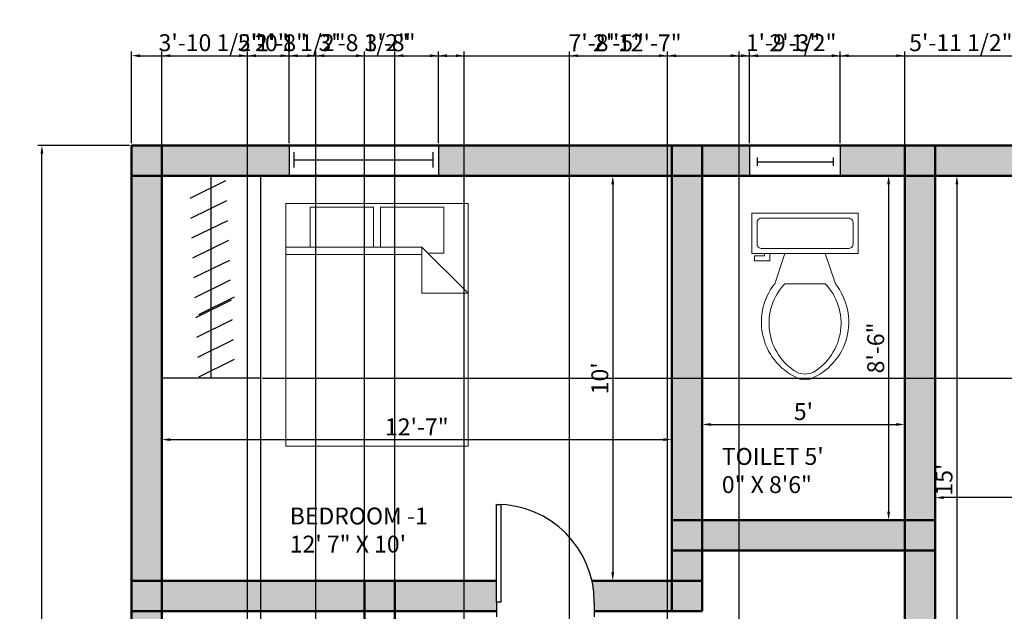
# Model space of a CAD drawing. Units: millimetres. Extents: x 2976 to 3516, y 849 to 1445.
# Tile 5 of 7: x 2981 to 3272, y 1270 to 1445. Entities that reach past the tile are written whole.
import ezdxf

# ---------------------------------------------------------------- set-up
doc = ezdxf.new("R2010")
doc.units = ezdxf.units.MM
for name, color, linetype, lineweight in [('A-AREA-IDEN', 150, 'Continuous', 25), ('A-FLOR-CASE', 130, 'Continuous', 25), ('A-FLOR-FIXT', 130, 'Continuous', 18), ('A-WALL-PATT', 3, 'Continuous', 13), ('dimensions', 50, 'Continuous', 18), ('doors', 190, 'Continuous', 25), ('furniture', 130, 'Continuous', 18), ('walls', 80, 'Continuous', 50), ('windows', 10, 'Continuous', 25)]:
    doc.layers.add(name, color=color, linetype=linetype, lineweight=lineweight)
doc.styles.get("Standard").update_dxf_attribs({"font": 'arial.ttf'})
doc.dimstyles.new('ISO-25', dxfattribs={"dimtxt": 5, "dimasz": 2.5, "dimexe": 1.25, "dimexo": 0.625, "dimtad": 1, "dimdec": 0, "dimlunit": 3, "dimtxsty": 'Standard', "dimcen": 2.5, "dimadec": 0, "dimazin": 0, "dimtfac": 1, "dimtdec": 0, "dimtmove": 0, "dimatfit": 3, "dimfxl": 1, "dimarcsym": 0})

# ---------------------------------------------------------------- blocks, each defined once
blk = doc.blocks.new('*U2')
for p, q in [((0, 0), (0, -6)), ((40, 0), (40, -6))]:
    blk.add_line(p, q)
blk.add_lwpolyline([(0, 0), (0, 40), (1.75, 40), (1.75, 0)], close=True)
blk.add_arc((0, 0), 40, 0, 90)
blk = doc.blocks.new('*U4')
for p, q in [((0, 4), (0, 0)), ((36, 4), (36, 0)), ((0, 2), (36, 2))]:
    blk.add_line(p, q)
blk = doc.blocks.new('*U5')
for p, q in [((0, 4), (0, 0)), ((0, 2), (36, 2)), ((36, 4), (36, 0))]:
    blk.add_line(p, q)
blk = doc.blocks.new('Bed - Queen')
for p, q in [((0, -80.00003), (0, 0)), ((0, 0), (59.99999, 0)), ((59.99999, 0), (59.99999, -80.00003)), ((7.99999, -1.2), (28.79998, -1.2)), ((7.99999, -14.4), (7.99999, -1.2)), ((28.79998, -1.2), (28.79998, -14.4)), ((31.19999, -1.2), (51.99999, -1.2)), ((31.19999, -14.4), (31.19999, -1.2)), ((51.99999, -1.2), (51.99999, -16.4)), ((0, -14.4), (44.8, -14.4)), ((59.99999, -29.6), (44.8, -14.4)), ((44.8, -14.4), (44.8, -29.6)), ((44.8, -16.8), (0, -16.8)), ((51.99999, -16.4), (46.79936, -16.4)), ((44.8, -29.6), (59.99999, -29.6)), ((59.99999, -80.00003), (0, -80.00003))]:
    blk.add_line(p, q)
blk = doc.blocks.new('Toilet - top')
for p, q in [((9.5, -6), (9.5, -2)), ((-10, -8.5), (-8, -8.5)), ((-10, -9.5), (-10, -8.5)), ((-7, -9.5), (-10, -9.5)), ((-8, -8.5), (-8, -8)), ((-7, -8), (-7, -9.5)), ((-4, -8), (-6, -14)), ((4, -8), (6, -14)), ((4, -14), (-4, -14))]:
    blk.add_line(p, q)
blk.add_lwpolyline([(10.5, -8), (10.5, 0), (-10.5, 0), (-10.5, -8)], close=True)
for points in [[(8.5, -1), (-8.5, -1)], [(-9.5, -2), (-9.5, -6)], [(-8.5, -7), (8.5, -7)]]:
    blk.add_lwpolyline(points)
for centre, radius, start, end in [((-8.62, -1.88), 0.884, 81.8699, 188.1301), ((8.62, -1.88), 0.884, 351.8699, 98.1301), ((-8.62, -6.12), 0.884, 171.8699, 278.1301), ((8.62, -6.12), 0.884, 261.8699, 8.1301), ((3.52, -21.58), 12.17, 141.4691, 247.9714), ((4.2, -21.82), 11.33, 136.3677, 238.9468), ((-3.52, -21.58), 12.17, 292.0284, 38.5307), ((-4.2, -21.82), 11.33, 301.053, 43.6321), ((0, -27.88), 4, 245.7318, 294.2682), ((0, -29), 4, 254.8605, 285.1395)]:
    blk.add_arc(centre, radius, start, end)
blk = doc.blocks.new('*D9')
at = {"layer": 'Defpoints', "color": 0, "transparency": 16777216}
for p in [(3156.2, 1398.88), (3156.2, 1278.88), (3156.2, 1278.88)]:
    blk.add_point(p, dxfattribs=at)
at = {"layer": 'dimensions', "color": 0, "lineweight": -2, "transparency": 16777216}
for p, q in [((3156.83, 1398.88), (3157.45, 1398.88)), ((3156.2, 1396.38), (3156.2, 1281.38)), ((3156.83, 1278.88), (3157.45, 1278.88))]:
    blk.add_line(p, q, dxfattribs=at)
at = {"layer": 'dimensions', "color": 0, "transparency": 16777216}
for points in [[(3155.78, 1396.38), (3156.62, 1396.38), (3156.2, 1398.88)], [(3155.78, 1281.38), (3156.62, 1281.38), (3156.2, 1278.88)]]:
    blk.add_solid(points, dxfattribs=at)
at = {"layer": 'dimensions', "color": 0, "transparency": 16777216, "insert": (3153.02, 1338.88), "char_height": 5, "attachment_point": 5, "rotation": 90}
blk.add_mtext("10'", dxfattribs=at)
blk = doc.blocks.new('*D10')
at = {"layer": 'Defpoints', "color": 0, "transparency": 16777216}
for p in [(3173.67, 1320.72), (3022.67, 1317.67), (3173.67, 1317.67)]:
    blk.add_point(p, dxfattribs=at)
at = {"layer": 'dimensions', "color": 0, "lineweight": -2, "transparency": 16777216}
for p, q in [((3022.67, 1318.3), (3022.67, 1321.97)), ((3173.67, 1318.3), (3173.67, 1321.97)), ((3025.17, 1320.72), (3171.17, 1320.72))]:
    blk.add_line(p, q, dxfattribs=at)
at = {"layer": 'dimensions', "color": 0, "transparency": 16777216}
for points in [[(3025.17, 1321.14), (3025.17, 1320.31), (3022.67, 1320.72)], [(3171.17, 1321.14), (3171.17, 1320.31), (3173.67, 1320.72)]]:
    blk.add_solid(points, dxfattribs=at)
at = {"layer": 'dimensions', "color": 0, "transparency": 16777216, "insert": (3098.17, 1323.86), "char_height": 5, "attachment_point": 5}
blk.add_mtext('12\'-7"', dxfattribs=at)
blk = doc.blocks.new('*D11')
at = {"layer": 'Defpoints', "color": 0, "transparency": 16777216}
for p in [(3237.91, 1398.88), (3237.91, 1296.88), (3237.91, 1296.88)]:
    blk.add_point(p, dxfattribs=at)
at = {"layer": 'dimensions', "color": 0, "lineweight": -2, "transparency": 16777216}
for p, q in [((3238.54, 1398.88), (3239.16, 1398.88)), ((3237.91, 1396.38), (3237.91, 1299.38)), ((3238.54, 1296.88), (3239.16, 1296.88))]:
    blk.add_line(p, q, dxfattribs=at)
at = {"layer": 'dimensions', "color": 0, "transparency": 16777216}
for points in [[(3237.49, 1396.38), (3238.33, 1396.38), (3237.91, 1398.88)], [(3237.49, 1299.38), (3238.33, 1299.38), (3237.91, 1296.88)]]:
    blk.add_solid(points, dxfattribs=at)
at = {"layer": 'dimensions', "color": 0, "transparency": 16777216, "insert": (3234.73, 1347.88), "char_height": 5, "attachment_point": 5, "rotation": 90}
blk.add_mtext('8\'-6"', dxfattribs=at)
blk = doc.blocks.new('*D12')
at = {"layer": 'Defpoints', "color": 0, "transparency": 16777216}
for p in [(3242.67, 1325.21), (3182.67, 1321.08), (3242.67, 1321.08)]:
    blk.add_point(p, dxfattribs=at)
at = {"layer": 'dimensions', "color": 0, "lineweight": -2, "transparency": 16777216}
for p, q in [((3182.67, 1321.71), (3182.67, 1326.46)), ((3185.17, 1325.21), (3240.17, 1325.21)), ((3242.67, 1321.71), (3242.67, 1326.46))]:
    blk.add_line(p, q, dxfattribs=at)
at = {"layer": 'dimensions', "color": 0, "transparency": 16777216}
for points in [[(3185.17, 1325.63), (3185.17, 1324.79), (3182.67, 1325.21)], [(3240.17, 1325.63), (3240.17, 1324.79), (3242.67, 1325.21)]]:
    blk.add_solid(points, dxfattribs=at)
at = {"layer": 'dimensions', "color": 0, "transparency": 16777216, "insert": (3212.67, 1328.38), "char_height": 5, "attachment_point": 5}
blk.add_mtext("5'", dxfattribs=at)
blk = doc.blocks.new('*D13')
at = {"layer": 'Defpoints', "color": 0, "transparency": 16777216}
for p in [(3251.67, 1303.56), (3251.67, 1303.56), (3383.67, 1303.56)]:
    blk.add_point(p, dxfattribs=at)
at = {"layer": 'dimensions', "color": 0, "lineweight": -2, "transparency": 16777216}
for p, q in [((3251.67, 1304.18), (3251.67, 1304.81)), ((3383.67, 1304.18), (3383.67, 1304.81)), ((3381.17, 1303.56), (3254.17, 1303.56))]:
    blk.add_line(p, q, dxfattribs=at)
at = {"layer": 'dimensions', "color": 0, "transparency": 16777216}
for points in [[(3254.17, 1303.98), (3254.17, 1303.14), (3251.67, 1303.56)], [(3381.17, 1303.98), (3381.17, 1303.14), (3383.67, 1303.56)]]:
    blk.add_solid(points, dxfattribs=at)
at = {"layer": 'dimensions', "color": 0, "transparency": 16777216, "insert": (3317.67, 1306.69), "char_height": 5, "attachment_point": 5}
blk.add_mtext("11'", dxfattribs=at)
blk = doc.blocks.new('*D14')
at = {"layer": 'Defpoints', "color": 0, "transparency": 16777216}
for p in [(3258.13, 1398.88), (3258.13, 1218.88), (3258.13, 1218.88)]:
    blk.add_point(p, dxfattribs=at)
at = {"layer": 'dimensions', "color": 0, "lineweight": -2, "transparency": 16777216}
for p, q in [((3258.76, 1398.88), (3259.38, 1398.88)), ((3258.13, 1396.38), (3258.13, 1221.38)), ((3258.76, 1218.88), (3259.38, 1218.88))]:
    blk.add_line(p, q, dxfattribs=at)
at = {"layer": 'dimensions', "color": 0, "transparency": 16777216}
for points in [[(3257.72, 1396.38), (3258.55, 1396.38), (3258.13, 1398.88)], [(3257.72, 1221.38), (3258.55, 1221.38), (3258.13, 1218.88)]]:
    blk.add_solid(points, dxfattribs=at)
at = {"layer": 'dimensions', "color": 0, "transparency": 16777216, "insert": (3254.96, 1308.88), "char_height": 5, "attachment_point": 5, "rotation": 90}
blk.add_mtext("15'", dxfattribs=at)
blk = doc.blocks.new('*D39')
at = {"layer": 'Defpoints', "color": 0, "transparency": 16777216}
for p in [(2987.13, 1407.88), (3013.67, 1407.88), (3013.67, 879.88)]:
    blk.add_point(p, dxfattribs=at)
at = {"layer": 'dimensions', "color": 0, "lineweight": -2, "transparency": 16777216}
for p, q in [((3013.05, 1407.88), (2985.88, 1407.88)), ((2987.13, 882.38), (2987.13, 1405.38)), ((3013.05, 879.88), (2985.88, 879.88))]:
    blk.add_line(p, q, dxfattribs=at)
at = {"layer": 'dimensions', "color": 0, "transparency": 16777216}
for points in [[(2986.71, 1405.38), (2987.55, 1405.38), (2987.13, 1407.88)], [(2986.71, 882.38), (2987.55, 882.38), (2987.13, 879.88)]]:
    blk.add_solid(points, dxfattribs=at)
at = {"layer": 'dimensions', "color": 0, "transparency": 16777216, "insert": (2983.95, 1143.88), "char_height": 5, "attachment_point": 5, "rotation": 90}
blk.add_mtext('44\'-0"', dxfattribs=at)
blk = doc.blocks.new('*D43')
at = {"layer": 'Defpoints', "color": 0, "transparency": 16777216}
for p in [(3082.67, 1434.42), (3022.67, 1140.88), (3082.67, 1140.88)]:
    blk.add_point(p, dxfattribs=at)
at = {"layer": 'dimensions', "color": 0, "lineweight": -2, "transparency": 16777216}
for p, q in [((3022.67, 1141.51), (3022.67, 1435.67)), ((3082.67, 1141.51), (3082.67, 1435.67)), ((3025.17, 1434.42), (3080.17, 1434.42))]:
    blk.add_line(p, q, dxfattribs=at)
at = {"layer": 'dimensions', "color": 0, "transparency": 16777216}
for points in [[(3025.17, 1434.84), (3025.17, 1434), (3022.67, 1434.42)], [(3080.17, 1434.84), (3080.17, 1434), (3082.67, 1434.42)]]:
    blk.add_solid(points, dxfattribs=at)
at = {"layer": 'dimensions', "color": 0, "transparency": 16777216, "insert": (3052.67, 1437.6), "char_height": 5, "attachment_point": 5}
blk.add_mtext('5\'-0"', dxfattribs=at)
blk = doc.blocks.new('*D44')
at = {"layer": 'Defpoints', "color": 0, "transparency": 16777216}
for p in [(3242.67, 1434.42), (3091.67, 1224.53), (3242.67, 1209.88)]:
    blk.add_point(p, dxfattribs=at)
at = {"layer": 'dimensions', "color": 0, "lineweight": -2, "transparency": 16777216}
for p, q in [((3091.67, 1225.16), (3091.67, 1435.67)), ((3242.67, 1210.51), (3242.67, 1435.67)), ((3094.17, 1434.42), (3240.17, 1434.42))]:
    blk.add_line(p, q, dxfattribs=at)
at = {"layer": 'dimensions', "color": 0, "transparency": 16777216}
for points in [[(3094.17, 1434.84), (3094.17, 1434), (3091.67, 1434.42)], [(3240.17, 1434.84), (3240.17, 1434), (3242.67, 1434.42)]]:
    blk.add_solid(points, dxfattribs=at)
at = {"layer": 'dimensions', "color": 0, "transparency": 16777216, "insert": (3167.17, 1437.56), "char_height": 5, "attachment_point": 5}
blk.add_mtext('12\'-7"', dxfattribs=at)
blk = doc.blocks.new('*D45')
at = {"layer": 'Defpoints', "color": 0, "transparency": 16777216}
for p in [(3060.33, 1434.42), (3013.67, 1407.88), (3060.33, 1407.88)]:
    blk.add_point(p, dxfattribs=at)
at = {"layer": 'dimensions', "color": 0, "lineweight": -2, "transparency": 16777216}
for p, q in [((3013.67, 1408.51), (3013.67, 1435.67)), ((3060.33, 1408.51), (3060.33, 1435.67)), ((3016.17, 1434.42), (3057.83, 1434.42))]:
    blk.add_line(p, q, dxfattribs=at)
at = {"layer": 'dimensions', "color": 0, "transparency": 16777216}
for points in [[(3016.17, 1434.84), (3016.17, 1434), (3013.67, 1434.42)], [(3057.83, 1434.84), (3057.83, 1434), (3060.33, 1434.42)]]:
    blk.add_solid(points, dxfattribs=at)
at = {"layer": 'dimensions', "color": 0, "transparency": 16777216, "insert": (3037, 1437.63), "char_height": 5, "attachment_point": 5}
blk.add_mtext('3\'-10 1/2"', dxfattribs=at)
blk = doc.blocks.new('*D46')
at = {"layer": 'Defpoints', "color": 0, "transparency": 16777216}
for p in [(3104.59, 1434.42), (3060.33, 1407.88), (3104.59, 1407.88)]:
    blk.add_point(p, dxfattribs=at)
at = {"layer": 'dimensions', "color": 0, "lineweight": -2, "transparency": 16777216}
for p, q in [((3060.33, 1408.51), (3060.33, 1435.67)), ((3104.59, 1408.51), (3104.59, 1435.67)), ((3062.83, 1434.42), (3102.09, 1434.42))]:
    blk.add_line(p, q, dxfattribs=at)
at = {"layer": 'dimensions', "color": 0, "transparency": 16777216}
for points in [[(3062.83, 1434.84), (3062.83, 1434), (3060.33, 1434.42)], [(3102.09, 1434.84), (3102.09, 1434), (3104.59, 1434.42)]]:
    blk.add_solid(points, dxfattribs=at)
at = {"layer": 'dimensions', "color": 0, "transparency": 16777216, "insert": (3082.46, 1437.63), "char_height": 5, "attachment_point": 5}
blk.add_mtext('3\'-8 1/2"', dxfattribs=at)
blk = doc.blocks.new('*D47')
at = {"layer": 'Defpoints', "color": 0, "transparency": 16777216}
for p in [(3196.7, 1434.42), (3104.59, 1407.88), (3196.7, 1407.88)]:
    blk.add_point(p, dxfattribs=at)
at = {"layer": 'dimensions', "color": 0, "lineweight": -2, "transparency": 16777216}
for p, q in [((3104.59, 1408.51), (3104.59, 1435.67)), ((3196.7, 1408.51), (3196.7, 1435.67)), ((3107.09, 1434.42), (3194.2, 1434.42))]:
    blk.add_line(p, q, dxfattribs=at)
at = {"layer": 'dimensions', "color": 0, "transparency": 16777216}
for points in [[(3107.09, 1434.84), (3107.09, 1434), (3104.59, 1434.42)], [(3194.2, 1434.84), (3194.2, 1434), (3196.7, 1434.42)]]:
    blk.add_solid(points, dxfattribs=at)
at = {"layer": 'dimensions', "color": 0, "transparency": 16777216, "insert": (3150.64, 1437.6), "char_height": 5, "attachment_point": 5}
blk.add_mtext('7\'-8"', dxfattribs=at)
blk = doc.blocks.new('*D48')
at = {"layer": 'Defpoints', "color": 0, "transparency": 16777216}
for p in [(3223.57, 1434.42), (3196.7, 1407.88), (3223.57, 1407.88)]:
    blk.add_point(p, dxfattribs=at)
at = {"layer": 'dimensions', "color": 0, "lineweight": -2, "transparency": 16777216}
for p, q in [((3196.7, 1408.51), (3196.7, 1435.67)), ((3223.57, 1408.51), (3223.57, 1435.67)), ((3199.2, 1434.42), (3221.07, 1434.42))]:
    blk.add_line(p, q, dxfattribs=at)
at = {"layer": 'dimensions', "color": 0, "transparency": 16777216}
for points in [[(3199.2, 1434.84), (3199.2, 1434), (3196.7, 1434.42)], [(3221.07, 1434.84), (3221.07, 1434), (3223.57, 1434.42)]]:
    blk.add_solid(points, dxfattribs=at)
at = {"layer": 'dimensions', "color": 0, "transparency": 16777216, "insert": (3210.14, 1437.6), "char_height": 5, "attachment_point": 5}
blk.add_mtext('2\'-3"', dxfattribs=at)
blk = doc.blocks.new('*D49')
at = {"layer": 'Defpoints', "color": 0, "transparency": 16777216}
for p in [(3295.02, 1434.42), (3223.57, 1407.88), (3295.02, 1407.88)]:
    blk.add_point(p, dxfattribs=at)
at = {"layer": 'dimensions', "color": 0, "lineweight": -2, "transparency": 16777216}
for p, q in [((3223.57, 1408.51), (3223.57, 1435.67)), ((3295.02, 1408.51), (3295.02, 1435.67)), ((3226.07, 1434.42), (3292.52, 1434.42))]:
    blk.add_line(p, q, dxfattribs=at)
at = {"layer": 'dimensions', "color": 0, "transparency": 16777216}
for points in [[(3226.07, 1434.84), (3226.07, 1434), (3223.57, 1434.42)], [(3292.52, 1434.84), (3292.52, 1434), (3295.02, 1434.42)]]:
    blk.add_solid(points, dxfattribs=at)
at = {"layer": 'dimensions', "color": 0, "transparency": 16777216, "insert": (3259.3, 1437.63), "char_height": 5, "attachment_point": 5}
blk.add_mtext('5\'-11 1/2"', dxfattribs=at)
blk = doc.blocks.new('*D54')
at = {"layer": 'Defpoints', "color": 0, "transparency": 16777216}
for p in [(3172.4, 1434.42), (3143.42, 1149.88), (3172.4, 1149.88)]:
    blk.add_point(p, dxfattribs=at)
at = {"layer": 'dimensions', "color": 0, "lineweight": -2, "transparency": 16777216}
for p, q in [((3143.42, 1150.51), (3143.42, 1435.67)), ((3172.4, 1150.51), (3172.4, 1435.67)), ((3145.92, 1434.42), (3169.9, 1434.42))]:
    blk.add_line(p, q, dxfattribs=at)
at = {"layer": 'dimensions', "color": 0, "transparency": 16777216}
for points in [[(3145.92, 1434.84), (3145.92, 1434), (3143.42, 1434.42)], [(3169.9, 1434.84), (3169.9, 1434), (3172.4, 1434.42)]]:
    blk.add_solid(points, dxfattribs=at)
at = {"layer": 'dimensions', "color": 0, "transparency": 16777216, "insert": (3157.91, 1437.6), "char_height": 5, "attachment_point": 5}
blk.add_mtext('2\'-5"', dxfattribs=at)
blk = doc.blocks.new('*D57')
at = {"layer": 'Defpoints', "color": 0, "transparency": 16777216}
for p in [(3112.23, 1434.42), (3068.25, 1017.88), (3112.23, 1017.88)]:
    blk.add_point(p, dxfattribs=at)
at = {"layer": 'dimensions', "color": 0, "lineweight": -2, "transparency": 16777216}
for p, q in [((3068.25, 1018.51), (3068.25, 1435.67)), ((3112.23, 1018.51), (3112.23, 1435.67)), ((3070.75, 1434.42), (3109.73, 1434.42))]:
    blk.add_line(p, q, dxfattribs=at)
at = {"layer": 'dimensions', "color": 0, "transparency": 16777216}
for points in [[(3070.75, 1434.84), (3070.75, 1434), (3068.25, 1434.42)], [(3109.73, 1434.84), (3109.73, 1434), (3112.23, 1434.42)]]:
    blk.add_solid(points, dxfattribs=at)
at = {"layer": 'dimensions', "color": 0, "transparency": 16777216, "insert": (3090.24, 1437.6), "char_height": 5, "attachment_point": 5}
blk.add_mtext('3\'-8"', dxfattribs=at)
blk = doc.blocks.new('*D73')
at = {"layer": 'Defpoints', "color": 0, "transparency": 16777216}
for p in [(3193.67, 1434.42), (3172.4, 1149.88), (3193.67, 1149.88)]:
    blk.add_point(p, dxfattribs=at)
at = {"layer": 'dimensions', "color": 0, "lineweight": -2, "transparency": 16777216}
for p, q in [((3172.4, 1150.51), (3172.4, 1435.67)), ((3193.67, 1150.51), (3193.67, 1435.67)), ((3174.9, 1434.42), (3191.17, 1434.42)), ((3193.67, 1434.42), (3221.89, 1434.42))]:
    blk.add_line(p, q, dxfattribs=at)
at = {"layer": 'dimensions', "color": 0, "transparency": 16777216}
for points in [[(3174.9, 1434.84), (3174.9, 1434), (3172.4, 1434.42)], [(3191.17, 1434.84), (3191.17, 1434), (3193.67, 1434.42)]]:
    blk.add_solid(points, dxfattribs=at)
at = {"layer": 'dimensions', "color": 0, "transparency": 16777216, "insert": (3209.03, 1437.63), "char_height": 5, "attachment_point": 5}
blk.add_mtext('1\'-9 1/2"', dxfattribs=at)
blk = doc.blocks.new('*D75')
at = {"layer": 'Defpoints', "color": 0, "transparency": 16777216}
for p in [(3022.67, 1338.88), (3051.83, 1338.88), (3051.83, 853.34)]:
    blk.add_point(p, dxfattribs=at)
at = {"layer": 'dimensions', "color": 0, "lineweight": -2, "transparency": 16777216}
for p, q in [((3022.67, 1338.26), (3022.67, 852.09)), ((3051.83, 1338.26), (3051.83, 852.09)), ((3025.17, 853.34), (3049.33, 853.34))]:
    blk.add_line(p, q, dxfattribs=at)
at = {"layer": 'dimensions', "color": 0, "transparency": 16777216}
for points in [[(3025.17, 853.76), (3025.17, 852.92), (3022.67, 853.34)], [(3049.33, 853.76), (3049.33, 852.92), (3051.83, 853.34)]]:
    blk.add_solid(points, dxfattribs=at)
at = {"layer": 'dimensions', "color": 0, "transparency": 16777216, "insert": (3037.25, 856.52), "char_height": 5, "attachment_point": 5}
blk.add_mtext('2\'-5"', dxfattribs=at)
blk = doc.blocks.new('*D76')
at = {"layer": 'Defpoints', "color": 0, "transparency": 16777216}
for p in [(3051.83, 1398.88), (3512.21, 1398.88), (3051.83, 1338.88)]:
    blk.add_point(p, dxfattribs=at)
at = {"layer": 'dimensions', "color": 0, "lineweight": -2, "transparency": 16777216}
for p, q in [((3052.46, 1398.88), (3513.46, 1398.88)), ((3512.21, 1341.38), (3512.21, 1396.38)), ((3052.46, 1338.88), (3513.46, 1338.88))]:
    blk.add_line(p, q, dxfattribs=at)
at = {"layer": 'dimensions', "color": 0, "transparency": 16777216}
for points in [[(3511.79, 1396.38), (3512.63, 1396.38), (3512.21, 1398.88)], [(3511.79, 1341.38), (3512.63, 1341.38), (3512.21, 1338.88)]]:
    blk.add_solid(points, dxfattribs=at)
at = {"layer": 'dimensions', "color": 0, "transparency": 16777216, "insert": (3509.03, 1368.88), "char_height": 5, "attachment_point": 5, "rotation": 90}
blk.add_mtext('5\'-0"', dxfattribs=at)
blk = doc.blocks.new('*D77')
at = {"layer": 'Defpoints', "color": 0, "transparency": 16777216}
for p in [(3048, 1434.42), (3022.67, 1079.38), (3048, 1079.38)]:
    blk.add_point(p, dxfattribs=at)
at = {"layer": 'dimensions', "color": 0, "lineweight": -2, "transparency": 16777216}
for p, q in [((3022.67, 1080.01), (3022.67, 1435.67)), ((3048, 1080.01), (3048, 1435.67)), ((3025.17, 1434.42), (3045.5, 1434.42)), ((3048, 1434.42), (3076.78, 1434.42))]:
    blk.add_line(p, q, dxfattribs=at)
at = {"layer": 'dimensions', "color": 0, "transparency": 16777216}
for points in [[(3025.17, 1434.84), (3025.17, 1434), (3022.67, 1434.42)], [(3045.5, 1434.84), (3045.5, 1434), (3048, 1434.42)]]:
    blk.add_solid(points, dxfattribs=at)
at = {"layer": 'dimensions', "color": 0, "transparency": 16777216, "insert": (3063.64, 1437.63), "char_height": 5, "attachment_point": 5}
blk.add_mtext('2\'-1 1/2"', dxfattribs=at)
blk = doc.blocks.new('*D79')
at = {"layer": 'Defpoints', "color": 0, "transparency": 16777216}
for p in [(3068.25, 1434.42), (3048, 1017.88), (3068.25, 1017.88)]:
    blk.add_point(p, dxfattribs=at)
at = {"layer": 'dimensions', "color": 0, "lineweight": -2, "transparency": 16777216}
for p, q in [((3048, 1018.51), (3048, 1435.67)), ((3068.25, 1018.51), (3068.25, 1435.67)), ((3050.5, 1434.42), (3065.75, 1434.42))]:
    blk.add_line(p, q, dxfattribs=at)
at = {"layer": 'dimensions', "color": 0, "transparency": 16777216}
for points in [[(3050.5, 1434.84), (3050.5, 1434), (3048, 1434.42)], [(3065.75, 1434.84), (3065.75, 1434), (3068.25, 1434.42)]]:
    blk.add_solid(points, dxfattribs=at)
at = {"layer": 'dimensions', "color": 0, "transparency": 16777216, "insert": (3058.12, 1437.6), "char_height": 5, "attachment_point": 5}
blk.add_mtext('1\'-8"', dxfattribs=at)

msp = doc.modelspace()

# ---------------------------------------------------------------- hatches: boundary and pattern name
at = {"layer": 'A-WALL-PATT'}
h = msp.add_hatch(color=256, dxfattribs=at)
h.dxf.hatch_style = 1
h.paths.add_polyline_path([(3022.67, 1398.88), (3013.67, 1398.88), (3013.67, 1278.88), (3022.67, 1278.88)])
h.paths.add_polyline_path([(3082.67, 1278.88), (3022.67, 1278.88), (3022.67, 1269.88), (3082.67, 1269.88)])
h.paths.add_polyline_path([(3022.67, 1278.88), (3013.67, 1278.88), (3013.67, 1269.88), (3022.67, 1269.88)])
h.paths.add_polyline_path([(3091.67, 1278.88), (3082.67, 1278.88), (3082.67, 1269.88), (3091.67, 1269.88)])
h.paths.add_polyline_path([(3121.76, 1278.88), (3091.67, 1278.88), (3091.67, 1269.88), (3121.76, 1269.88), (3121.76, 1272.56)])
h.paths.add_polyline_path([(3022.67, 1269.88), (3013.67, 1269.88), (3013.67, 1149.88), (3022.67, 1149.88)])
h.paths.add_polyline_path([(3022.67, 1140.88), (3013.67, 1140.88), (3013.67, 1017.88), (3022.67, 1017.88)])
h.paths.add_polyline_path([(3022.67, 1149.88), (3013.67, 1149.88), (3013.67, 1140.88), (3022.67, 1140.88)])
h.paths.add_polyline_path([(3082.67, 1149.88), (3022.67, 1149.88), (3022.67, 1140.88), (3082.67, 1140.88)])
h.paths.add_polyline_path([(3091.67, 1149.88), (3082.67, 1149.88), (3082.67, 1140.88), (3091.67, 1140.88)])
h.paths.add_polyline_path([(3143.42, 1147.68), (3143.42, 1149.88), (3091.67, 1149.88), (3091.67, 1140.88), (3144.23, 1140.88, -0.059251)])
h.paths.add_polyline_path([(3193.67, 1149.88), (3172.4, 1149.88), (3172.4, 1147.68), (3172.4, 1140.88), (3193.67, 1140.88)])
h.paths.add_polyline_path([(3202.67, 1149.88), (3193.67, 1149.88), (3193.67, 1140.88), (3202.67, 1140.88)])
h.paths.add_polyline_path([(3272.67, 1149.88), (3262.67, 1149.88), (3262.67, 1140.88), (3272.67, 1140.88)])
h.paths.add_polyline_path([(3272.67, 1140.88), (3262.67, 1140.88), (3262.67, 1083.88), (3272.67, 1083.88)])
h.paths.add_polyline_path([(3202.67, 1140.88), (3193.67, 1140.88), (3193.67, 1090.58), (3195.4, 1090.58, -0.118064), (3202.67, 1088.84)])
h.paths.add_polyline_path([(3202.67, 1074.53), (3195.4, 1074.53), (3193.67, 1074.53), (3193.67, 1017.88), (3202.67, 1017.88)])
h.paths.add_polyline_path([(3202.67, 1017.88), (3193.67, 1017.88), (3193.67, 1008.88), (3202.67, 1008.88)])
h.paths.add_polyline_path([(3193.67, 1017.88), (3112.23, 1017.88), (3112.23, 1008.88), (3193.67, 1008.88)])
h.paths.add_polyline_path([(3068.25, 1017.88), (3022.67, 1017.88), (3022.67, 1008.88), (3068.25, 1008.88)])
h.paths.add_polyline_path([(3022.67, 1017.88), (3013.67, 1017.88), (3013.67, 1008.88), (3022.67, 1008.88)])
h.paths.add_polyline_path([(3272.67, 1074.88), (3262.67, 1074.88), (3262.67, 1017.88), (3271.67, 1017.88), (3272.67, 1017.88)])
h.paths.add_polyline_path([(3272.67, 1083.88), (3262.67, 1083.88), (3262.67, 1074.88), (3272.67, 1074.88)])
h.paths.add_polyline_path([(3284.41, 1082.91), (3284.41, 1083.88), (3272.67, 1083.88), (3272.67, 1074.88), (3284.41, 1074.88)])
h.paths.add_polyline_path([(3383.67, 1083.88), (3300.46, 1083.88), (3300.46, 1082.91, -0.131652), (3298.31, 1074.88), (3383.67, 1074.88)])
h.paths.add_polyline_path([(3392.67, 1083.88), (3383.67, 1083.88), (3383.67, 1074.88), (3392.67, 1074.88)])
h.paths.add_polyline_path([(3392.67, 1074.88), (3383.67, 1074.88), (3383.67, 1017.88), (3392.67, 1017.88)])
h.paths.add_polyline_path([(3392.67, 1017.88), (3383.67, 1017.88), (3383.67, 1008.88), (3392.67, 1008.88)])
h.paths.add_polyline_path([(3383.67, 1017.88), (3347.17, 1017.88), (3347.17, 1008.88), (3383.67, 1008.88)])
h.paths.add_polyline_path([(3303.78, 1017.88), (3272.67, 1017.88), (3272.67, 1008.88), (3303.78, 1008.88)])
h.paths.add_polyline_path([(3272.67, 1017.88), (3271.67, 1017.88), (3262.67, 1017.88), (3262.67, 1008.88), (3272.67, 1008.88)])
h.paths.add_polyline_path([(3262.67, 1017.88), (3243.44, 1017.88), (3243.44, 1008.88), (3262.67, 1008.88)])
h.paths.add_polyline_path([(3218.58, 1017.88), (3202.67, 1017.88), (3202.67, 1008.88), (3218.58, 1008.88)])
h.paths.add_polyline_path([(3392.67, 1209.88), (3383.67, 1209.88), (3383.67, 1083.88), (3392.67, 1083.88)])
h.paths.add_polyline_path([(3392.67, 1218.88), (3383.67, 1218.88), (3383.67, 1209.88), (3392.67, 1209.88)])
h.paths.add_polyline_path([(3392.67, 1246.1), (3383.67, 1246.1), (3383.67, 1218.88), (3392.67, 1218.88)])
h.paths.add_polyline_path([(3383.67, 1218.88), (3251.67, 1218.88), (3251.67, 1209.88), (3383.67, 1209.88)])
h.paths.add_polyline_path([(3251.67, 1287.88), (3242.67, 1287.88), (3242.67, 1218.88), (3251.67, 1218.88)])
h.paths.add_polyline_path([(3251.67, 1218.88), (3242.67, 1218.88), (3242.67, 1209.88), (3251.67, 1209.88)])
h.paths.add_polyline_path([(3251.67, 1398.88), (3242.67, 1398.88), (3242.67, 1296.88), (3251.67, 1296.88)])
h.paths.add_polyline_path([(3251.67, 1296.88), (3242.67, 1296.88), (3242.67, 1287.88), (3251.67, 1287.88)])
h.paths.add_polyline_path([(3242.67, 1296.88), (3182.67, 1296.88), (3182.67, 1287.88), (3242.67, 1287.88)])
h.paths.add_polyline_path([(3182.67, 1296.88), (3173.67, 1296.88), (3173.67, 1287.88), (3182.67, 1287.88)])
h.paths.add_polyline_path([(3182.67, 1287.88), (3173.67, 1287.88), (3173.67, 1278.88), (3182.67, 1278.88)])
h.paths.add_polyline_path([(3182.67, 1278.88), (3173.67, 1278.88), (3173.67, 1269.88), (3182.67, 1269.88)])
h.paths.add_polyline_path([(3173.67, 1278.88), (3150.05, 1278.88, -0.054989), (3150.74, 1272.56), (3150.74, 1269.88), (3173.67, 1269.88)])
h.paths.add_polyline_path([(3182.67, 1398.88), (3173.67, 1398.88), (3173.67, 1296.88), (3182.67, 1296.88)])
h.paths.add_polyline_path([(3182.67, 1407.88), (3173.67, 1407.88), (3173.67, 1398.88), (3182.67, 1398.88)])
h.paths.add_polyline_path([(3173.67, 1407.88), (3104.59, 1407.88), (3104.59, 1398.88), (3173.67, 1398.88)])
h.paths.add_polyline_path([(3060.33, 1407.88), (3022.67, 1407.88), (3022.67, 1398.88), (3060.33, 1398.88)])
h.paths.add_polyline_path([(3022.67, 1407.88), (3013.67, 1407.88), (3013.67, 1398.88), (3022.67, 1398.88)])
h.paths.add_polyline_path([(3196.7, 1407.88), (3182.67, 1407.88), (3182.67, 1398.88), (3196.7, 1398.88)])
h.paths.add_polyline_path([(3242.67, 1407.88), (3223.57, 1407.88), (3223.57, 1398.88), (3242.67, 1398.88)])
h.paths.add_polyline_path([(3251.67, 1407.88), (3242.67, 1407.88), (3242.67, 1398.88), (3251.67, 1398.88)])
h.paths.add_polyline_path([(3295.02, 1407.88), (3251.67, 1407.88), (3251.67, 1398.88), (3295.02, 1398.88)])
h.paths.add_polyline_path([(3383.67, 1407.88), (3338.5, 1407.88), (3338.5, 1398.88), (3383.67, 1398.88)])
h.paths.add_polyline_path([(3392.67, 1407.88), (3383.67, 1407.88), (3383.67, 1398.88), (3392.67, 1398.88)])
h.paths.add_polyline_path([(3392.67, 1398.88), (3383.67, 1398.88), (3383.67, 1273.3, -0.079613), (3392.67, 1275.07)])

# ---------------------------------------------------------------- linework, layer by layer
at = {"layer": 'A-FLOR-CASE'}
for p, q in [((3041.51, 1397.33), (3030.9, 1392.12)), ((3037.25, 1338.88), (3037.25, 1398.88)), ((3041.79, 1391.45), (3031.18, 1386.24)), ((3042.08, 1385.57), (3031.47, 1380.36)), ((3042.36, 1379.69), (3031.75, 1374.48)), ((3042.65, 1373.81), (3032.04, 1368.6)), ((3042.93, 1367.93), (3032.32, 1362.72)), ((3043.22, 1362.05), (3032.61, 1356.84)), ((3044.07, 1362.89), (3033.46, 1357.69)), ((3043.5, 1356.17), (3032.89, 1350.96)), ((3043.78, 1350.29), (3033.18, 1345.08)), ((3044.07, 1344.41), (3033.46, 1339.2)), ((3051.83, 1338.88), (3022.67, 1338.88))]:
    msp.add_line(p, q, dxfattribs=at)
msp.add_lwpolyline([(3022.67, 1398.88), (3051.83, 1398.88), (3051.83, 1278.88), (3022.67, 1278.88)], close=True, dxfattribs=at)
at = {"layer": 'walls'}
for p, q in [((3013.67, 1407.88), (3013.67, 1008.88)), ((3013.67, 1407.88), (3392.67, 1407.88)), ((3022.67, 1407.88), (3022.67, 1008.88)), ((3173.67, 1407.88), (3173.67, 1269.88)), ((3182.67, 1407.88), (3182.67, 1269.88)), ((3242.67, 1407.88), (3242.67, 1209.88)), ((3251.67, 1407.88), (3251.67, 1209.88)), ((3013.67, 1398.88), (3392.67, 1398.88)), ((3173.67, 1296.88), (3251.67, 1296.88)), ((3173.67, 1287.88), (3251.67, 1287.88)), ((3013.67, 1278.88), (3121.76, 1278.88)), ((3082.67, 1278.88), (3082.67, 1140.88)), ((3091.67, 1278.88), (3091.67, 1140.88)), ((3150.05, 1278.88), (3182.67, 1278.88)), ((3013.67, 1269.88), (3121.76, 1269.88)), ((3150.74, 1269.88), (3182.67, 1269.88))]:
    msp.add_line(p, q, dxfattribs=at)
at = {"layer": 'windows'}
for p, q in [((3060.33, 1407.88), (3060.33, 1398.88)), ((3104.59, 1407.88), (3104.59, 1398.88)), ((3196.7, 1407.88), (3196.7, 1398.88)), ((3223.57, 1407.88), (3223.57, 1398.88))]:
    msp.add_line(p, q, dxfattribs=at)

# ---------------------------------------------------------------- block references
at = {"layer": 'A-FLOR-FIXT', "xscale": 1.496177724149161, "yscale": 1.496177724149161, "zscale": 1.496177724149161}
msp.add_blockref('Toilet - top', (3213.15, 1387.84), dxfattribs=at)
at = {"layer": 'doors', "xscale": 0.7246062005204927, "yscale": 0.7246062005204927, "zscale": 0.7246062005204927}
msp.add_blockref('*U2', (3121.76, 1272.56), dxfattribs=at)
at = {"layer": 'furniture', "xscale": 0.8990276149147879, "yscale": 0.8990276149147879, "zscale": 0.8990276149147879}
msp.add_blockref('Bed - Queen', (3059.41, 1390.67), dxfattribs=at)
at = {"layer": 'windows'}
for name, p, xscale, yscale, zscale in [('*U4', (3061.77, 1401.32), 1.141608635997284, 1.141608635997284, 1.141608635997284), ('*U5', (3198.99, 1401.78), 0.6246542558083853, 0.6246542558083853, 0.6246542558083853)]:
    msp.add_blockref(name, p, dxfattribs=dict(at, xscale=xscale, yscale=yscale, zscale=zscale))

# ---------------------------------------------------------------- texts
at = {"layer": 'A-AREA-IDEN', "char_height": 5, "attachment_point": 1}
for s, width, insert in [('TOILET 5\' 0" X 8\'6"', 36.4499, (3188.51, 1318.24)), ('BEDROOM -1\\P12\' 7" X 10\'', 52.8837, (3060.53, 1300.61))]:
    msp.add_mtext_dynamic_manual_height_columns(s, width=width, gutter_width=12.5, heights=[0], dxfattribs=dict(at, insert=insert))

# ---------------------------------------------------------------- dimensions: what is measured, and where the dimension line sits
at = {"layer": 'dimensions'}
for base, p1, p2, override, picture, middle in [((3060.33, 1434.42), (3013.67, 1407.88), (3060.33, 1407.88), {"dimdec": 1, "dimlfac": 1, "dimrnd": 0, "dimzin": 1, "dimdsep": 46, "dimlunit": 4, "dimfrac": 2}, '*D45', (3037, 1437.63)), ((3048, 1434.42), (3022.67, 1079.38), (3048, 1079.38), {"dimdec": 1, "dimlfac": 1, "dimrnd": 0, "dimzin": 1, "dimdsep": 46, "dimlunit": 4, "dimfrac": 2}, '*D77', (3063.64, 1437.63)), ((3104.59, 1434.42), (3060.33, 1407.88), (3104.59, 1407.88), {"dimdec": 1, "dimlfac": 1, "dimrnd": 0, "dimzin": 1, "dimdsep": 46, "dimlunit": 4, "dimfrac": 2}, '*D46', (3082.46, 1437.63)), ((3193.67, 1434.42), (3172.4, 1149.88), (3193.67, 1149.88), {"dimdec": 1, "dimlfac": 1, "dimrnd": 0, "dimzin": 1, "dimdsep": 46, "dimlunit": 4, "dimfrac": 2}, '*D73', (3209.03, 1437.63)), ((3295.0222, 1434.4215), (3223.5747, 1407.8815), (3295.0222, 1407.8815), {"dimdec": 1, "dimlfac": 1, "dimrnd": 0, "dimzin": 1, "dimdsep": 46, "dimlunit": 4, "dimfrac": 2}, '*D49', (3259.2985, 1437.6317)), ((3082.67, 1434.42), (3022.67, 1140.88), (3082.67, 1140.88), {"dimdec": 1, "dimlfac": 1, "dimrnd": 0, "dimzin": 1, "dimdsep": 46, "dimlunit": 4, "dimfrac": 2}, '*D43', (3052.67, 1437.6)), ((3068.248, 1434.4215), (3047.9988, 1017.8815), (3068.248, 1017.8815), {"dimdec": 1, "dimlfac": 1, "dimrnd": 0, "dimzin": 1, "dimdsep": 46, "dimlunit": 4, "dimfrac": 2}, '*D79', (3058.1234, 1437.5993)), ((3112.23, 1434.42), (3068.25, 1017.88), (3112.23, 1017.88), {"dimdec": 1, "dimlfac": 1, "dimrnd": 0, "dimzin": 1, "dimdsep": 46, "dimlunit": 4, "dimfrac": 2}, '*D57', (3090.24, 1437.6)), ((3242.67, 1434.42), (3091.67, 1224.53), (3242.67, 1209.88), {"dimdec": 1, "dimlfac": 1, "dimrnd": 0, "dimzin": 1, "dimdsep": 46, "dimlunit": 4, "dimfrac": 2}, '*D44', (3167.17, 1437.56)), ((3196.7, 1434.42), (3104.59, 1407.88), (3196.7, 1407.88), {"dimdec": 1, "dimlfac": 1, "dimrnd": 0, "dimzin": 1, "dimdsep": 46, "dimlunit": 4, "dimfrac": 2}, '*D47', (3150.64, 1437.6)), ((3172.4, 1434.42), (3143.42, 1149.88), (3172.4, 1149.88), {"dimdec": 1, "dimlfac": 1, "dimrnd": 0, "dimzin": 1, "dimdsep": 46, "dimlunit": 4, "dimfrac": 2}, '*D54', (3157.91, 1437.6)), ((3223.57, 1434.42), (3196.7, 1407.88), (3223.57, 1407.88), {"dimdec": 1, "dimlfac": 1, "dimrnd": 0, "dimzin": 1, "dimdsep": 46, "dimlunit": 4, "dimfrac": 2}, '*D48', (3210.14, 1437.6)), ((3051.83, 853.34), (3022.67, 1338.88), (3051.83, 1338.88), {"dimdec": 1, "dimlfac": 1, "dimrnd": 0, "dimzin": 1, "dimdsep": 46, "dimlunit": 4, "dimfrac": 2}, '*D75', (3037.25, 856.52)), ((3242.67, 1325.21), (3182.67, 1321.08), (3242.67, 1321.08), {"dimclrd": 0, "dimclre": 0, "dimclrt": 0}, '*D12', (3212.67, 1328.38)), ((3173.67, 1320.72), (3022.67, 1317.67), (3173.67, 1317.67), {"dimclrd": 0, "dimclre": 0, "dimclrt": 0}, '*D10', (3098.17, 1323.86)), ((3251.67, 1303.56), (3383.67, 1303.56), (3251.67, 1303.56), {"dimclrd": 0, "dimclre": 0, "dimclrt": 0}, '*D13', (3317.67, 1306.69))]:
    dim = msp.add_linear_dim(base=base, p1=p1, p2=p2, dimstyle='ISO-25', override=override, dxfattribs=at)
    dim.commit()
    dim.dimension.update_dxf_attribs({"geometry": picture, "text_midpoint": middle})
for base, p1, p2, override, picture, middle in [((2987.13, 1407.88), (3013.67, 879.88), (3013.67, 1407.88), {"dimdec": 1, "dimlfac": 1, "dimrnd": 0, "dimzin": 1, "dimdsep": 46, "dimlunit": 4, "dimfrac": 2}, '*D39', (2983.95, 1143.88)), ((3512.21, 1398.88), (3051.83, 1338.88), (3051.83, 1398.88), {"dimdec": 1, "dimlfac": 1, "dimrnd": 0, "dimzin": 1, "dimdsep": 46, "dimlunit": 4, "dimfrac": 2}, '*D76', (3509.03, 1368.88)), ((3156.2, 1278.88), (3156.2, 1398.88), (3156.2, 1278.88), {"dimclrd": 0, "dimclre": 0, "dimclrt": 0}, '*D9', (3153.02, 1338.88)), ((3237.91, 1296.88), (3237.91, 1398.88), (3237.91, 1296.88), {"dimclrd": 0, "dimclre": 0, "dimclrt": 0}, '*D11', (3234.73, 1347.88)), ((3258.13, 1218.88), (3258.13, 1398.88), (3258.13, 1218.88), {"dimclrd": 0, "dimclre": 0, "dimclrt": 0}, '*D14', (3254.96, 1308.88))]:
    dim = msp.add_linear_dim(base=base, p1=p1, p2=p2, angle=90, dimstyle='ISO-25', override=override, dxfattribs=at)
    dim.commit()
    dim.dimension.update_dxf_attribs({"geometry": picture, "text_midpoint": middle})

doc.saveas('drawing.dxf')
